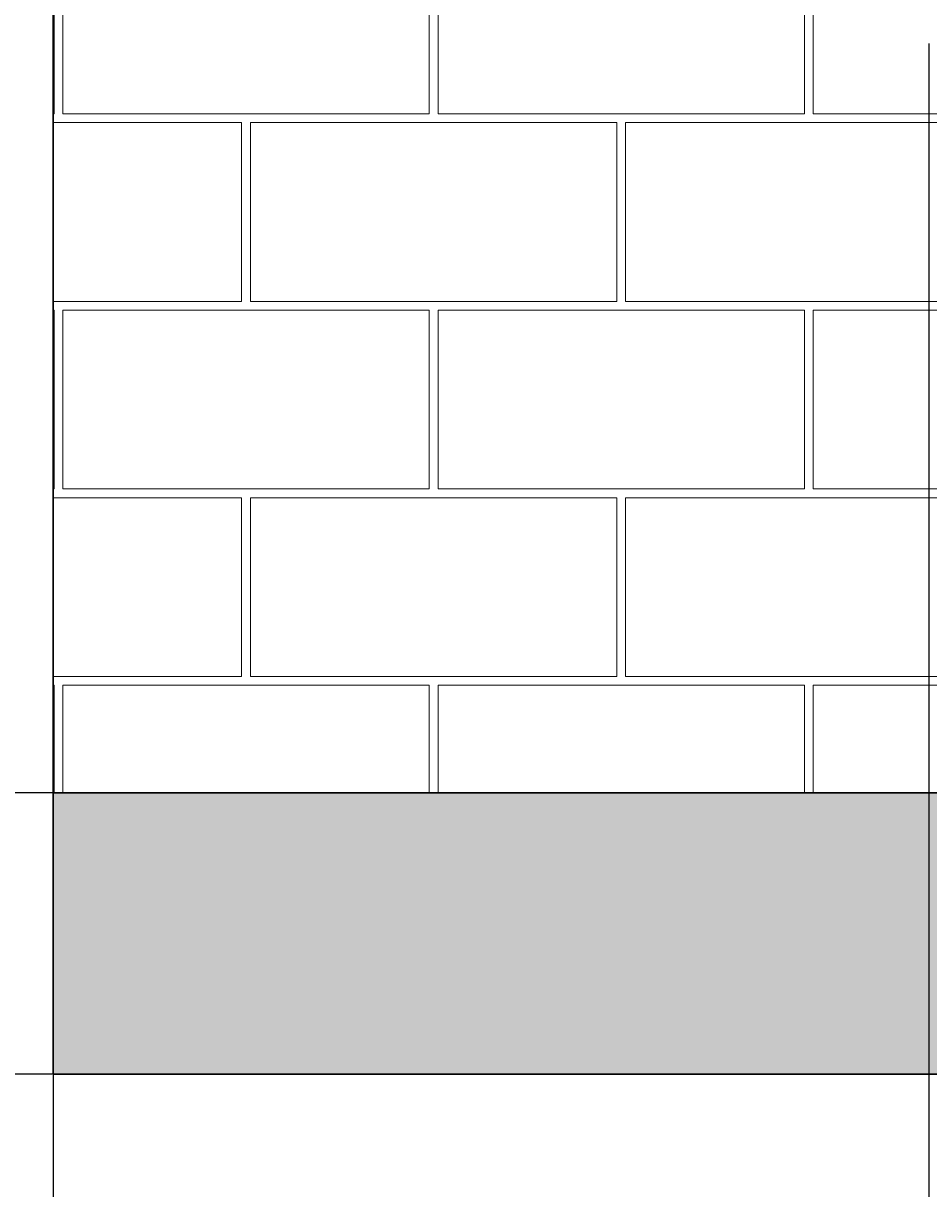
# Model space of a CAD drawing. Units: inches. Extents: x -301 to 715, y -607 to 364.
# Tile 128 of 141: x 252 to 310, y -515 to -440. Entities that reach past the tile are written whole.
import ezdxf

# ---------------------------------------------------------------- set-up
doc = ezdxf.new("R2010")
doc.units = ezdxf.units.IN
doc.header["$MEASUREMENT"] = 0
for name, color, linetype, lineweight in [('A-ANNO-DIMS', 2, 'Continuous', 18), ('A-ELEV', 220, 'Continuous', 30), ('A-ELEV-PATT', 4, 'Continuous', 13), ('A-GRND', 7, 'Continuous', 25)]:
    doc.layers.add(name, color=color, linetype=linetype, lineweight=lineweight)
doc.styles.get("Standard").update_dxf_attribs({"font": 'arial.ttf'})
doc.dimstyles.get("Standard").update_dxf_attribs({"dimtxt": 0.18, "dimasz": 0.18, "dimexe": 0.18, "dimexo": 0.0625, "dimgap": 0.09, "dimtad": 0, "dimtih": 1, "dimtoh": 1, "dimdec": 1, "dimzin": 0, "dimdsep": 46, "dimlunit": 4, "dimtxsty": 'Standard', "dimcen": 0.09, "dimclrd": 3, "dimclre": 4, "dimclrt": 6, "dimadec": 0, "dimazin": 0, "dimtfac": 1, "dimtdec": 1, "dimtofl": 0, "dimtmove": 0, "dimatfit": 3, "dimfxl": 1, "dimtfill": 2, "dimtfillclr": 51, "dimtolj": 1, "dimtzin": 0, "dimarcsym": 0})

# ---------------------------------------------------------------- blocks, each defined once
blk = doc.blocks.new('*D194')
at = {"layer": 'A-ANNO-DIMS', "color": 4, "lineweight": -2, "transparency": 16777216}
for p, q in [((310.018, -441.615), (310.018, -606.789)), ((254.018, -507.615), (254.018, -606.789))]:
    blk.add_line(p, q, dxfattribs=at)
at = {"layer": 'A-ANNO-DIMS', "color": 3, "lineweight": -2, "transparency": 16777216}
for p, q in [((254.198, -606.609), (281.685, -606.609)), ((309.838, -606.609), (282.351, -606.609))]:
    blk.add_line(p, q, dxfattribs=at)
at = {"layer": 'A-ANNO-DIMS', "color": 3, "transparency": 16777216}
for points in [[(254.198, -606.579), (254.198, -606.639), (254.018, -606.609)], [(309.838, -606.579), (309.838, -606.639), (310.018, -606.609)]]:
    blk.add_solid(points, dxfattribs=at)
at = {"layer": 'Defpoints', "color": 0, "transparency": 16777216}
for p in [(310.018, -441.552), (254.018, -507.552), (310.018, -606.609)]:
    blk.add_point(p, dxfattribs=at)
at = {"layer": 'A-ANNO-DIMS', "color": 6, "transparency": 16777216, "insert": (282.018, -606.609), "char_height": 0.18, "attachment_point": 5, "bg_fill": 1, "box_fill_scale": 1.25, "bg_fill_color": 51, "bg_fill_transparency": 0}
blk.add_mtext('\\A1;4\'-8"', dxfattribs=at)
blk = doc.blocks.new('*D195')
at = {"layer": 'A-ANNO-DIMS', "color": 4, "lineweight": -2, "transparency": 16777216}
for p, q in [((310.018, -441.615), (310.018, -606.789)), ((360.018, -441.615), (360.018, -606.789))]:
    blk.add_line(p, q, dxfattribs=at)
at = {"layer": 'A-ANNO-DIMS', "color": 3, "lineweight": -2, "transparency": 16777216}
for p, q in [((310.198, -606.609), (334.685, -606.609)), ((359.838, -606.609), (335.351, -606.609))]:
    blk.add_line(p, q, dxfattribs=at)
at = {"layer": 'A-ANNO-DIMS', "color": 3, "transparency": 16777216}
for points in [[(310.198, -606.579), (310.198, -606.639), (310.018, -606.609)], [(359.838, -606.579), (359.838, -606.639), (360.018, -606.609)]]:
    blk.add_solid(points, dxfattribs=at)
at = {"layer": 'Defpoints', "color": 0, "transparency": 16777216}
for p in [(310.018, -441.552), (360.018, -441.552), (360.018, -606.609)]:
    blk.add_point(p, dxfattribs=at)
at = {"layer": 'A-ANNO-DIMS', "color": 6, "transparency": 16777216, "insert": (335.018, -606.609), "char_height": 0.18, "attachment_point": 5, "bg_fill": 1, "box_fill_scale": 1.25, "bg_fill_color": 51, "bg_fill_transparency": 0}
blk.add_mtext('\\A1;4\'-2"', dxfattribs=at)
blk = doc.blocks.new('*D200')
at = {"layer": 'A-ANNO-DIMS', "color": 4, "lineweight": -2, "transparency": 16777216}
for p, q in [((412.955, -393.552), (121.926, -393.552)), ((412.955, -489.552), (121.926, -489.552))]:
    blk.add_line(p, q, dxfattribs=at)
at = {"layer": 'A-ANNO-DIMS', "color": 3, "lineweight": -2, "transparency": 16777216}
for p, q in [((122.106, -393.732), (122.106, -441.371)), ((122.106, -489.372), (122.106, -441.734))]:
    blk.add_line(p, q, dxfattribs=at)
at = {"layer": 'A-ANNO-DIMS', "color": 3, "transparency": 16777216}
for points in [[(122.076, -393.732), (122.136, -393.732), (122.106, -393.552)], [(122.076, -489.372), (122.136, -489.372), (122.106, -489.552)]]:
    blk.add_solid(points, dxfattribs=at)
at = {"layer": 'Defpoints', "color": 0, "transparency": 16777216}
for p in [(122.106, -393.552), (413.018, -393.552), (413.018, -489.552)]:
    blk.add_point(p, dxfattribs=at)
at = {"layer": 'A-ANNO-DIMS', "color": 6, "transparency": 16777216, "insert": (122.106, -441.552), "char_height": 0.18, "attachment_point": 5, "bg_fill": 1, "box_fill_scale": 1.25, "bg_fill_color": 51, "bg_fill_transparency": 0}
blk.add_mtext('\\A1;8\'-0"', dxfattribs=at)

msp = doc.modelspace()

# ---------------------------------------------------------------- hatches: boundary and pattern name
at = {"layer": 'A-ELEV-PATT'}
h = msp.add_hatch(dxfattribs=at)
h.set_pattern_fill('AR-B816C', color=256, scale=1.5)
h.set_pattern_definition([(0, (458.621, 9.325), (12, 12), [23.4375, -0.5625]), (0, (446.621, 9.887), (12, 12), [23.4375, -0.5625]), (90, (458.621, 9.325), (-12, 12), [-12.5625, 11.4375]), (90, (458.059, 9.325), (-12, 12), [-12.5625, 11.4375])])
h.paths.add_polyline_path([(254.018, -489.552), (413.018, -489.552), (413.018, -393.552), (461.018, -393.552), (461.018, -489.552), (591.518, -489.552), (591.518, -369.552), (254.018, -369.552)])
h.paths.add_polyline_path([(310.018, -393.552), (360.018, -393.552), (360.018, -441.552), (310.018, -441.552)], flags=16)
h.paths.add_polyline_path([(315.018, -398.552), (355.018, -398.552), (355.018, -436.552), (315.018, -436.552)], flags=0)
h.paths.add_polyline_path([(496.768, -393.552), (546.768, -393.552), (546.768, -441.552), (496.768, -441.552)], flags=16)
h.paths.add_polyline_path([(501.768, -398.552), (541.768, -398.552), (541.768, -436.552), (501.768, -436.552)], flags=0)
h = msp.add_hatch(dxfattribs=at)
h.set_pattern_fill('AR-CONC', color=256, scale=2)
h.set_pattern_definition([(50, (458.621, 9.325), (14.3452, -1.25504), [1.5, -16.5]), (355, (458.621, 9.325), (-2.77503, 15.04384), [1.2, -13.2]), (100.4514, (459.817, 9.22), (11.57018, 13.7888), [1.2748, -14.02284]), (46.1842, (458.621, 13.325), (21.3448, -3.3104), [2.25, -24.75]), (96.6356, (460.4, 13.049), (18.69324, 19.4824), [1.9122, -21.0343]), (351.184, (458.62, 13.325), (18.6932, 19.4824), [1.8, -19.8]), (21, (460.621, 12.325), (11.93814, -8.05238), [1.5, -16.5]), (326, (460.621, 12.325), (4.8663, 14.503), [1.2, -13.2]), (71.4514, (461.616, 11.654), (16.80445, 6.45062), [1.2748, -14.02284]), (37.5, (458.621, 9.325), (0.243197, 6.657877), [0, -13.04, 0, -13.4, 0, -13.25]), (7.5, (458.621, 9.325), (5.26139, 7.88823), [0, -7.64, 0, -12.74, 0, -5.05]), (327.5, (454.161, 9.325), (10.67645, -0.4511), [0, -5, 0, -15.6, 0, -20.7]), (317.5, (452.161, 9.325), (11.66372, 2.0021), [0, -6.5, 0, -10.36, 0, -14.7])])
h.paths.add_polyline_path([(254.018, -489.552), (254.018, -507.552), (413.018, -507.552), (413.018, -489.552)])
h.paths.add_polyline_path([(591.518, -507.552), (591.518, -489.552), (461.018, -489.552), (461.018, -507.552)])

# ---------------------------------------------------------------- linework, layer by layer
at = {"layer": 'A-ELEV'}
for p, q in [((254.018, -489.552), (591.518, -489.552)), ((254.018, -507.552), (591.518, -507.552))]:
    msp.add_line(p, q, dxfattribs=at)
for points in [[(254.018, -369.552), (591.518, -369.552), (591.518, -489.552), (254.018, -489.552)], [(254.018, -489.552), (591.518, -489.552), (591.518, -507.552), (254.018, -507.552)]]:
    msp.add_lwpolyline(points, close=True, dxfattribs=at)
at = {"layer": 'A-GRND'}
msp.add_line((254.018, -507.552), (206.018, -507.552), dxfattribs=at)

# ---------------------------------------------------------------- dimensions: what is measured, and where the dimension line sits
at = {"layer": 'A-ANNO-DIMS'}
dim = msp.add_linear_dim(base=(122.106, -393.552), p1=(413.018, -489.552), p2=(413.018, -393.552), angle=90, dimstyle='Standard', override={"dimdec": 1, "dimlfac": 1, "dimrnd": 0, "dimzin": 1, "dimdsep": 46, "dimlunit": 4, "dimfrac": 2}, dxfattribs=at)
dim.commit()
dim.dimension.update_dxf_attribs({"geometry": '*D200', "text_midpoint": (122.106, -441.552)})
for base, p1, p2, picture, middle in [((310.018, -606.609), (254.018, -507.552), (310.018, -441.552), '*D194', (282.018, -606.609)), ((360.018, -606.609), (310.018, -441.552), (360.018, -441.552), '*D195', (335.018, -606.609))]:
    dim = msp.add_linear_dim(base=base, p1=p1, p2=p2, dimstyle='Standard', override={"dimdec": 1, "dimlfac": 1, "dimrnd": 0, "dimzin": 1, "dimdsep": 46, "dimlunit": 4, "dimfrac": 2}, dxfattribs=at)
    dim.commit()
    dim.dimension.update_dxf_attribs({"geometry": picture, "text_midpoint": middle})

doc.saveas('drawing.dxf')
